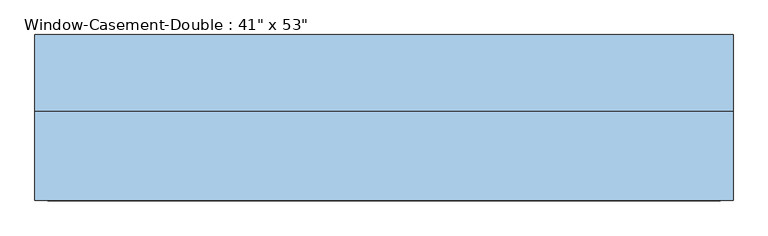
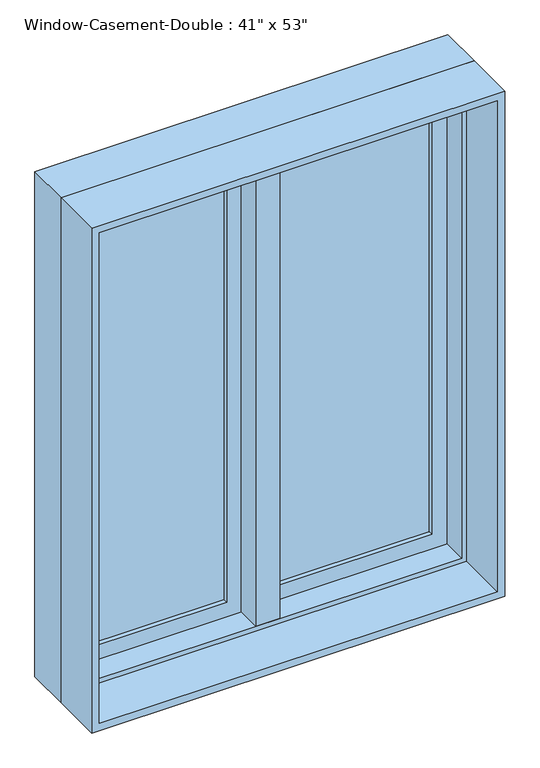
"""IFC4 building model written with IfcOpenShell, lengths in millimetres: window geometry."""

from ifc_helpers import new_model, si_unit, frame, origin, place, context, project, spatial, polyline, outline, extrude, faceted_brep, source, transform, mapped, element, save


def window_c95ebb39(model_context):
    return source(origin(), model_context, "Body", "SolidModel", [
        faceted_brep([(9.525, 133.35, 2247.9), (-9.525, 133.35, 2247.9), (-9.525, 82.55, 2247.9), (9.525, 82.55, 2247.9), (9.525, 133.35, 927.1), (9.525, 82.55, 927.1), (-9.525, 82.55, 927.1), (-9.525, 133.35, 927.1), (-9.525, 82.55, 946.15), (-9.525, 82.55, 2228.85), (-30.1625, 82.55, 946.15), (-30.1625, 82.55, 2228.85), (-30.1625, 19.05, 946.15), (-30.1625, 19.05, 2228.85), (30.1625, 19.05, 946.15), (30.1625, 19.05, 2228.85), (30.1625, 82.55, 946.15), (30.1625, 82.55, 2228.85), (9.525, 82.55, 946.15), (9.525, 82.55, 2228.85)], [[[0, 1, 2, 3]], [[4, 5, 6, 7]], [[1, 0, 4, 7]], [[2, 1, 7, 6, 8, 9]], [[9, 8, 10, 11]], [[11, 10, 12, 13]], [[13, 12, 14, 15]], [[15, 14, 16, 17]], [[17, 16, 18, 19]], [[0, 3, 19, 18, 5, 4]], [[18, 8, 6, 5]], [[9, 19, 3, 2]], [[8, 18, 16, 14, 12, 10]], [[19, 9, 11, 13, 15, 17]]]),
        extrude(outline(polyline([(-66.675, 114.3), (-66.675, 107.95), (-450.85, 107.95), (-450.85, 114.3), (-66.675, 114.3)])), frame((0.0, 0.0, 984.25), z_axis=(0.0, 0.0, 1.0), x_axis=(1.0, 0.0, 0.0)), (0.0, 0.0, 1.0), 1206.5),
        extrude(outline(polyline([(-450.85, 95.25), (-450.85, 101.6), (-66.675, 101.6), (-66.675, 95.25), (-450.85, 95.25)])), frame((0.0, 0.0, 984.25), z_axis=(0.0, 0.0, 1.0), x_axis=(1.0, 0.0, 0.0)), (0.0, 0.0, 1.0), 1206.5),
        extrude(outline(polyline([(450.85, 114.3), (450.85, 107.95), (66.675, 107.95), (66.675, 114.3), (450.85, 114.3)])), frame((0.0, 0.0, 984.25), z_axis=(0.0, 0.0, 1.0), x_axis=(1.0, 0.0, 0.0)), (0.0, 0.0, 1.0), 1206.5),
        extrude(outline(polyline([(66.675, 95.25), (66.675, 101.6), (450.85, 101.6), (450.85, 95.25), (66.675, 95.25)])), frame((0.0, 0.0, 984.25), z_axis=(0.0, 0.0, 1.0), x_axis=(1.0, 0.0, 0.0)), (0.0, 0.0, 1.0), 1206.5),
        extrude(outline(polyline([(2247.9, -508.0), (927.1, -508.0), (927.1, -9.525), (2247.9, -9.525), (2247.9, -508.0)]), holes=[polyline([(2190.75, -66.675), (984.25, -66.675), (984.25, -450.85), (2190.75, -450.85), (2190.75, -66.675)])]), frame((0.0, 82.55, 0.0), z_axis=(0.0, 1.0, 0.0), x_axis=(0.0, 0.0, 1.0)), (0.0, 0.0, 1.0), 44.45),
        extrude(outline(polyline([(927.1, 508.0), (2247.9, 508.0), (2247.9, 9.525), (927.1, 9.525), (927.1, 508.0)]), holes=[polyline([(984.25, 66.675), (2190.75, 66.675), (2190.75, 450.85), (984.25, 450.85), (984.25, 66.675)])]), frame((0.0, 82.55, 0.0), z_axis=(0.0, 1.0, 0.0), x_axis=(0.0, 0.0, 1.0)), (0.0, 0.0, 1.0), 44.45),
        extrude(outline(polyline([(2260.6, -520.7), (914.4, -520.7), (914.4, 520.7), (2260.6, 520.7), (2260.6, -520.7)]), holes=[polyline([(2241.55, 501.65), (933.45, 501.65), (933.45, -501.65), (2241.55, -501.65), (2241.55, 501.65)])]), frame((0.0, -114.3, 0.0), z_axis=(0.0, 1.0, 0.0), x_axis=(0.0, 0.0, 1.0)), (0.0, 0.0, 1.0), 133.35),
        faceted_brep([(488.95, 82.55, 2228.85), (488.95, 19.05, 2228.85), (-488.95, 19.05, 2228.85), (-488.95, 82.55, 2228.85), (508.0, 133.35, 2247.9), (508.0, 82.55, 2247.9), (-508.0, 82.55, 2247.9), (-508.0, 133.35, 2247.9), (520.7, 19.05, 2260.6), (520.7, 133.35, 2260.6), (-520.7, 133.35, 2260.6), (-520.7, 19.05, 2260.6), (-488.95, 19.05, 946.15), (-488.95, 82.55, 946.15), (-508.0, 82.55, 927.1), (-508.0, 133.35, 927.1), (-520.7, 133.35, 914.4), (-520.7, 19.05, 914.4), (488.95, 19.05, 946.15), (488.95, 82.55, 946.15), (508.0, 82.55, 927.1), (508.0, 133.35, 927.1), (520.7, 133.35, 914.4), (520.7, 19.05, 914.4)], [[[0, 1, 2, 3]], [[4, 5, 6, 7]], [[8, 9, 10, 11]], [[3, 2, 12, 13]], [[7, 6, 14, 15]], [[11, 10, 16, 17]], [[13, 12, 18, 19]], [[15, 14, 20, 21]], [[17, 16, 22, 23]], [[11, 17, 23, 8], [1, 18, 12, 2]], [[19, 18, 1, 0]], [[5, 20, 14, 6], [3, 13, 19, 0]], [[21, 20, 5, 4]], [[23, 22, 9, 8]], [[9, 22, 16, 10], [7, 15, 21, 4]]]),
    ])


if __name__ == "__main__":
    model = new_model("IFC4")
    model_context = context("Model", 3, world=origin())
    ifc_project = project(units=[si_unit("LENGTHUNIT", "METRE", prefix="MILLI")], contexts=[model_context])
    site = spatial("IfcSite", under=ifc_project)
    building = spatial("IfcBuilding", under=site)
    placement = place(None, origin())
    window_shape = window_c95ebb39(model_context)
    element("IfcWindow", 1, ObjectType="Window-Casement-Double : 41\" x 53\"", at=placement, inside=building, context=model_context, shape_type="MappedRepresentation", body=[
        mapped(window_shape, transform((0.0, 0.0, 0.0), x_axis=(1.0, 0.0, 0.0), y_axis=(0.0, 1.0, 0.0), z_axis=(0.0, 0.0, 1.0))),
    ])
    save(model, "model.ifc")

# Revit data of these elements
# Type "Window-Casement-Double : 41\" x 53\""
#   Type Mark = "15"
#   Fire Rating = "0.5h"
#   Assembly Code = "B2020100"
#   Analytic Construction = "Double glazing - domestic"
#   Frame Extension [instance default] = 0' - 0 1/4"
#   Window Inset [instance default] = 0' - 0"
#   Wall Thickness [instance default] = 0' - 6"
#   Interior Wall Closure [instance default] = 0' - 2 1/4"
#   Half Width = 1' - 8 1/2"
#   Visual Light Transmittance = 0.81
#   Thermal Resistance (R) = 1.8146 (h·ft²·°F)/BTU
#   Solar Heat Gain Coefficient = 0.76
#   Rough Width = 3' - 5 1/2"
#   Rough Height = 4' - 5 1/2"
#   Height = 4' - 5"
#   Heat Transfer Coefficient (U) = 0.5511 BTU/(h·ft²·°F)
#   Exterior Wall Closure [instance default] = 0' - 1 1/4"
#   Extension Jamb [instance default] = 0' - 2 1/4"
#   Default Sill Height = 3' - 0"
#   Width = 3' - 5"
#   Define Thermal Properties by = 0
#   Muntin Visibility = yes
#   Interior Trim Visibility [instance default] = yes
#   Exterior Trim Visibility [instance default] = yes
#   Extension Jamb Visibility [instance default] = yes
#   Interior Trim Material = Wood - Stained
#   Muntin Pattern = Muntin Pattern_2x2 : Muntin Pattern_2x2
#   Interior Trim = Trim-Window-Interior-Flat : Picture Frame
#   Interior Frame Material = Wood - Stained
#   Glass Panel Material = Glass
#   Exterior Trim Material = Clad - White
#   Exterior Trim = Trim-Window-Exterior-Flat : with Sill
#   Exterior Frame Material = Clad - White
#   Wall Closure = (empty or 0)
# Element 1 (IfcWindow, "Window-Casement-Double : 41\" x 53\"")
#   Wall Thickness = 0' - 9"
#   Extension Jamb = 0' - 5 1/4"
#   Materials on its faces: "Wood - Stained", "Glass", "Clad - White"
# Materials
#   "Wood - Stained": class "Wood", colour RGB 224 178 126, transparency 0, Cost = 0
#   "Glass": class "Glass", colour RGB 0 128 192, transparency 0.75, Description = "Soda Lime Glass", Cost = 0
#   "Clad - White": class "Wood", colour RGB 242 242 238, transparency 0, Cost = 0
